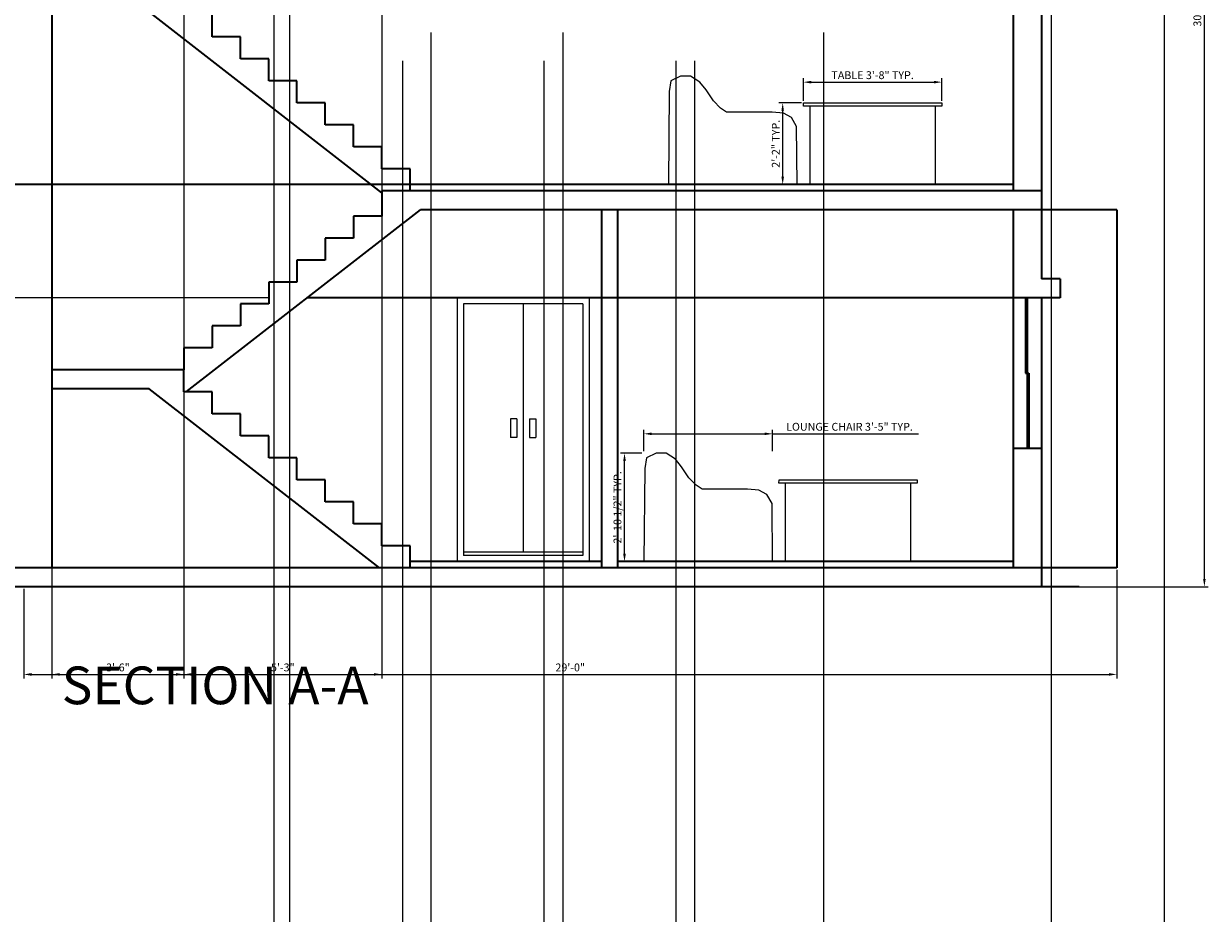
# Model space of a CAD drawing. Units: inches. Extents: x 2443635 to 2446153, y 1826255 to 1827341.
# Tile 13 of 16: x 2445143 to 2445520, y 1826759 to 1827042. Entities that reach past the tile are written whole.
import ezdxf

# ---------------------------------------------------------------- set-up
doc = ezdxf.new("R2010")
doc.units = ezdxf.units.IN
for name, color, linetype, lineweight in [('A-ANNO-LEVL', 4, 'Continuous', 18), ('A-DIMS', 1, 'Continuous', 18), ('A-FURN', 6, 'Continuous', 18), ('A-REFR', 8, 'Continuous', 13), ('A-SECT', 7, 'Continuous', 35), ('A-SECT-PROJ', 9, 'Continuous', 18), ('A-TEXT', 4, 'Continuous', 25)]:
    doc.layers.add(name, color=color, linetype=linetype, lineweight=lineweight)
doc.styles.get("Standard").update_dxf_attribs({"font": 'arial.ttf'})
doc.dimstyles.new('ISO-25', dxfattribs={"dimtxt": 2.5, "dimasz": 2.5, "dimexe": 1.25, "dimexo": 0.625, "dimtad": 1, "dimlunit": 4, "dimtxsty": 'Standard', "dimcen": 2.5, "dimadec": 0, "dimazin": 0, "dimtfac": 1, "dimtmove": 0, "dimatfit": 3, "dimfxl": 1, "dimarcsym": 0})

# ---------------------------------------------------------------- blocks, each defined once
blk = doc.blocks.new('TABLE-SECTION')
at = {"transparency": 33554687}
for p, q in [((2.02, 25), (2.02, 0)), ((42.02, 0), (42.02, 25)), ((2.02, 0), (42.02, 0))]:
    blk.add_line(p, q, dxfattribs=at)
blk.add_lwpolyline([(42.02, 25), (2.02, 25), (0, 25), (0.02, 26), (44.02, 26), (44.06, 25)], close=True, dxfattribs=at)
blk = doc.blocks.new('LOUNGE-CHAIR-SECTION')
at = {"transparency": 33554687}
blk.add_lwpolyline([(0, 0.15), (41.01, 0), (40.81, 18.51), (39.18, 21.33), (36.62, 22.78), (33.02, 23.03), (18.53, 23.09), (16.64, 24.31), (14.33, 26.66), (12.01, 30.12), (10.03, 32.62), (7.07, 34.53), (3.89, 34.53), (0.84, 32.99), (0.3, 29.59), (0.04, 0.15)], dxfattribs=at)
blk = doc.blocks.new('*D74')
at = {"layer": 'A-DIMS', "color": 0, "lineweight": -2, "transparency": 16777216}
for p, q in [((2445391.11, 1827017.33), (2445391.11, 1827024.56)), ((2445435.17, 1827017.33), (2445435.17, 1827024.56)), ((2445393.61, 1827023.31), (2445432.67, 1827023.31))]:
    blk.add_line(p, q, dxfattribs=at)
at = {"layer": 'A-DIMS', "color": 0, "transparency": 16777216}
for points in [[(2445393.61, 1827023.73), (2445393.61, 1827022.89), (2445391.11, 1827023.31)], [(2445432.67, 1827023.73), (2445432.67, 1827022.89), (2445435.17, 1827023.31)]]:
    blk.add_solid(points, dxfattribs=at)
at = {"layer": 'Defpoints', "color": 0, "transparency": 16777216}
for p in [(2445435.17, 1827023.31), (2445391.11, 1827016.7), (2445435.17, 1827016.7)]:
    blk.add_point(p, dxfattribs=at)
at = {"layer": 'A-DIMS', "color": 0, "transparency": 16777216, "insert": (2445413.14, 1827025.21), "char_height": 2.5, "attachment_point": 5}
blk.add_mtext('TABLE 3\'-8" TYP.', dxfattribs=at)
blk = doc.blocks.new('*D75')
at = {"layer": 'A-DIMS', "color": 0, "lineweight": -2, "transparency": 16777216}
for p, q in [((2445390.49, 1827016.7), (2445383.26, 1827016.7)), ((2445384.51, 1826993.2), (2445384.51, 1827014.2)), ((2445390.49, 1826990.7), (2445383.26, 1826990.7))]:
    blk.add_line(p, q, dxfattribs=at)
at = {"layer": 'A-DIMS', "color": 0, "transparency": 16777216}
for points in [[(2445384.09, 1827014.2), (2445384.92, 1827014.2), (2445384.51, 1827016.7)], [(2445384.09, 1826993.2), (2445384.92, 1826993.2), (2445384.51, 1826990.7)]]:
    blk.add_solid(points, dxfattribs=at)
at = {"layer": 'Defpoints', "color": 0, "transparency": 16777216}
for p in [(2445384.51, 1827016.7), (2445391.11, 1827016.7), (2445391.11, 1826990.7)]:
    blk.add_point(p, dxfattribs=at)
at = {"layer": 'A-DIMS', "color": 0, "transparency": 16777216, "insert": (2445382.63, 1827003.7), "char_height": 2.5, "attachment_point": 5, "rotation": 90}
blk.add_mtext('2\'-2" TYP.', dxfattribs=at)
blk = doc.blocks.new('*D88')
at = {"layer": 'A-DIMS', "color": 0, "lineweight": -2, "transparency": 16777216}
for p, q in [((2445340.3, 1826905.86), (2445340.3, 1826912.63)), ((2445342.8, 1826911.38), (2445378.81, 1826911.38)), ((2445381.31, 1826905.86), (2445381.31, 1826912.63)), ((2445381.31, 1826911.38), (2445427.75, 1826911.38))]:
    blk.add_line(p, q, dxfattribs=at)
at = {"layer": 'A-DIMS', "color": 0, "transparency": 16777216}
for points in [[(2445342.8, 1826911.8), (2445342.8, 1826910.97), (2445340.3, 1826911.38)], [(2445378.81, 1826911.8), (2445378.81, 1826910.97), (2445381.31, 1826911.38)]]:
    blk.add_solid(points, dxfattribs=at)
at = {"layer": 'Defpoints', "color": 0, "transparency": 16777216}
for p in [(2445381.31, 1826911.38), (2445340.3, 1826905.23), (2445381.31, 1826905.23)]:
    blk.add_point(p, dxfattribs=at)
at = {"layer": 'A-DIMS', "color": 0, "transparency": 16777216, "insert": (2445405.78, 1826913.3), "char_height": 2.5, "attachment_point": 5}
blk.add_mtext('LOUNGE CHAIR 3\'-5" TYP.', dxfattribs=at)
blk = doc.blocks.new('*D89')
at = {"layer": 'A-DIMS', "color": 0, "lineweight": -2, "transparency": 16777216}
for p, q in [((2445339.68, 1826905.23), (2445332.9, 1826905.23)), ((2445334.15, 1826873.2), (2445334.15, 1826902.73)), ((2445339.68, 1826870.7), (2445332.9, 1826870.7))]:
    blk.add_line(p, q, dxfattribs=at)
at = {"layer": 'A-DIMS', "color": 0, "transparency": 16777216}
for points in [[(2445333.73, 1826902.73), (2445334.57, 1826902.73), (2445334.15, 1826905.23)], [(2445333.73, 1826873.2), (2445334.57, 1826873.2), (2445334.15, 1826870.7)]]:
    blk.add_solid(points, dxfattribs=at)
at = {"layer": 'Defpoints', "color": 0, "transparency": 16777216}
for p in [(2445334.15, 1826905.23), (2445340.3, 1826905.23), (2445340.3, 1826870.7)]:
    blk.add_point(p, dxfattribs=at)
at = {"layer": 'A-DIMS', "color": 0, "transparency": 16777216, "insert": (2445332.23, 1826887.97), "char_height": 2.5, "attachment_point": 5, "rotation": 90}
blk.add_mtext('2\'-10 1/2" TYP.', dxfattribs=at)
blk = doc.blocks.new('*D99')
at = {"layer": 'A-DIMS', "color": 0, "lineweight": -2, "transparency": 16777216}
for p, q in [((2445286.12, 1827228.7), (2445520.01, 1827228.7)), ((2445518.76, 1826865.2), (2445518.76, 1827226.2)), ((2445143.49, 1826862.7), (2445520.01, 1826862.7))]:
    blk.add_line(p, q, dxfattribs=at)
at = {"layer": 'A-DIMS', "color": 0, "transparency": 16777216}
for points in [[(2445518.35, 1827226.2), (2445519.18, 1827226.2), (2445518.76, 1827228.7)], [(2445518.35, 1826865.2), (2445519.18, 1826865.2), (2445518.76, 1826862.7)]]:
    blk.add_solid(points, dxfattribs=at)
at = {"layer": 'Defpoints', "color": 0, "transparency": 16777216}
for p in [(2445285.49, 1827228.7), (2445518.76, 1827228.7), (2445142.86, 1826862.7)]:
    blk.add_point(p, dxfattribs=at)
at = {"layer": 'A-DIMS', "color": 0, "transparency": 16777216, "insert": (2445516.86, 1827045.7), "char_height": 2.5, "attachment_point": 5, "rotation": 90}
blk.add_mtext('30\'-6"', dxfattribs=at)
blk = doc.blocks.new('*D100')
at = {"layer": 'A-DIMS', "color": 0, "lineweight": -2, "transparency": 16777216}
for p, q in [((2445490.86, 1826868.08), (2445490.86, 1826833.55)), ((2445142.86, 1826862.08), (2445142.86, 1826833.55)), ((2445145.36, 1826834.8), (2445488.36, 1826834.8))]:
    blk.add_line(p, q, dxfattribs=at)
at = {"layer": 'A-DIMS', "color": 0, "transparency": 16777216}
for points in [[(2445145.36, 1826835.22), (2445145.36, 1826834.38), (2445142.86, 1826834.8)], [(2445488.36, 1826835.22), (2445488.36, 1826834.38), (2445490.86, 1826834.8)]]:
    blk.add_solid(points, dxfattribs=at)
at = {"layer": 'Defpoints', "color": 0, "transparency": 16777216}
for p in [(2445490.86, 1826868.7), (2445142.86, 1826862.7), (2445490.86, 1826834.8)]:
    blk.add_point(p, dxfattribs=at)
at = {"layer": 'A-DIMS', "color": 0, "transparency": 16777216, "insert": (2445316.86, 1826836.7), "char_height": 2.5, "attachment_point": 5}
blk.add_mtext('29\'-0"', dxfattribs=at)
blk = doc.blocks.new('*D102')
at = {"layer": 'A-DIMS', "color": 0, "lineweight": -2, "transparency": 16777216}
for p, q in [((2445151.86, 1827051.08), (2445151.86, 1826833.55)), ((2445193.86, 1827051.08), (2445193.86, 1826833.55)), ((2445154.36, 1826834.8), (2445191.36, 1826834.8))]:
    blk.add_line(p, q, dxfattribs=at)
at = {"layer": 'A-DIMS', "color": 0, "transparency": 16777216}
for points in [[(2445154.36, 1826835.22), (2445154.36, 1826834.38), (2445151.86, 1826834.8)], [(2445191.36, 1826835.22), (2445191.36, 1826834.38), (2445193.86, 1826834.8)]]:
    blk.add_solid(points, dxfattribs=at)
at = {"layer": 'Defpoints', "color": 0, "transparency": 16777216}
for p in [(2445151.86, 1827051.7), (2445193.86, 1827051.7), (2445193.86, 1826834.8)]:
    blk.add_point(p, dxfattribs=at)
at = {"layer": 'A-DIMS', "color": 0, "transparency": 16777216, "insert": (2445172.86, 1826836.7), "char_height": 2.5, "attachment_point": 5}
blk.add_mtext('3\'-6"', dxfattribs=at)
blk = doc.blocks.new('*D103')
at = {"layer": 'A-DIMS', "color": 0, "lineweight": -2, "transparency": 16777216}
for p, q in [((2445256.86, 1827108.08), (2445256.86, 1826833.55)), ((2445193.86, 1827051.08), (2445193.86, 1826833.55)), ((2445196.36, 1826834.8), (2445254.36, 1826834.8))]:
    blk.add_line(p, q, dxfattribs=at)
at = {"layer": 'A-DIMS', "color": 0, "transparency": 16777216}
for points in [[(2445196.36, 1826835.22), (2445196.36, 1826834.38), (2445193.86, 1826834.8)], [(2445254.36, 1826835.22), (2445254.36, 1826834.38), (2445256.86, 1826834.8)]]:
    blk.add_solid(points, dxfattribs=at)
at = {"layer": 'Defpoints', "color": 0, "transparency": 16777216}
for p in [(2445256.86, 1827108.7), (2445193.86, 1827051.7), (2445256.86, 1826834.8)]:
    blk.add_point(p, dxfattribs=at)
at = {"layer": 'A-DIMS', "color": 0, "transparency": 16777216, "insert": (2445225.36, 1826836.7), "char_height": 2.5, "attachment_point": 5}
blk.add_mtext('5\'-3"', dxfattribs=at)

msp = doc.modelspace()

# ---------------------------------------------------------------- linework, layer by layer
at = {"layer": 'A-ANNO-LEVL'}
msp.add_line((2445220.864, 1826954.701), (2445021.398, 1826954.701), dxfattribs=at)
at = {"layer": 'A-REFR'}
for p, q in [((2445469.966, 1827104.133), (2445469.966, 1826329.288)), ((2445505.966, 1827104.133), (2445505.966, 1826329.288)), ((2445272.466, 1827039.133), (2445272.466, 1826255.288)), ((2445314.466, 1827039.133), (2445314.466, 1826255.288)), ((2445397.466, 1827039.133), (2445397.466, 1826264.288)), ((2445263.466, 1827030.133), (2445263.466, 1826255.288)), ((2445308.466, 1827030.133), (2445308.466, 1826255.288)), ((2445350.466, 1827030.133), (2445350.466, 1826255.288)), ((2445356.466, 1827030.133), (2445356.466, 1826255.288))]:
    msp.add_line(p, q, dxfattribs=at)
at = {"layer": 'A-REFR', "transparency": 33554687}
for p in [(2445227.466, 1827321.207), (2445222.466, 1827316.303)]:
    msp.add_ray(p, (0, -1), dxfattribs=at)
at = {"layer": 'A-SECT'}
for p, q in [((2445151.864, 1827222.701), (2445151.864, 1826868.701)), ((2445457.864, 1827102.701), (2445457.864, 1826988.701)), ((2445466.864, 1827102.701), (2445466.864, 1826982.701)), ((2445256.864, 1826988.1), (2445182.805, 1827045.701)), ((2445202.864, 1827037.701), (2445202.864, 1827044.701)), ((2445211.864, 1827037.701), (2445202.864, 1827037.701)), ((2445211.864, 1827030.701), (2445211.864, 1827037.701)), ((2445220.864, 1827030.701), (2445211.864, 1827030.701)), ((2445220.864, 1827023.701), (2445220.864, 1827030.701)), ((2445229.864, 1827023.701), (2445220.864, 1827023.701)), ((2445229.864, 1827016.701), (2445229.864, 1827023.701)), ((2445238.864, 1827016.701), (2445229.864, 1827016.701)), ((2445238.864, 1827009.701), (2445238.864, 1827016.701)), ((2445247.864, 1827009.701), (2445238.864, 1827009.701)), ((2445247.864, 1827002.701), (2445247.864, 1827009.701)), ((2445256.864, 1827002.701), (2445247.864, 1827002.701)), ((2445256.864, 1826995.701), (2445256.864, 1827002.701)), ((2445265.864, 1826995.701), (2445256.864, 1826995.701)), ((2445265.864, 1826988.701), (2445265.864, 1826995.701)), ((2445457.864, 1826990.701), (2445021.398, 1826990.701)), ((2445466.864, 1826988.701), (2445256.864, 1826988.701)), ((2445256.864, 1826988.701), (2445256.864, 1826980.701)), ((2445194.637, 1826924.701), (2445269.208, 1826982.701)), ((2445490.864, 1826982.701), (2445269.208, 1826982.701)), ((2445326.864, 1826982.701), (2445326.864, 1826868.701)), ((2445331.864, 1826982.701), (2445331.864, 1826868.701)), ((2445457.864, 1826982.701), (2445457.864, 1826868.701)), ((2445466.864, 1826982.701), (2445466.864, 1826960.701)), ((2445490.864, 1826982.701), (2445490.864, 1826868.701)), ((2445256.864, 1826980.701), (2445247.864, 1826980.701)), ((2445247.864, 1826980.701), (2445247.864, 1826973.701)), ((2445247.864, 1826973.701), (2445238.864, 1826973.701)), ((2445238.864, 1826973.701), (2445238.864, 1826966.701)), ((2445238.864, 1826966.701), (2445229.864, 1826966.701)), ((2445229.864, 1826966.701), (2445229.864, 1826959.701)), ((2445472.864, 1826960.701), (2445466.864, 1826960.701)), ((2445472.864, 1826960.701), (2445472.864, 1826954.701)), ((2445229.864, 1826959.701), (2445220.864, 1826959.701)), ((2445220.864, 1826959.701), (2445220.864, 1826952.701)), ((2445220.864, 1826952.701), (2445211.864, 1826952.701)), ((2445211.864, 1826952.701), (2445211.864, 1826945.701)), ((2445457.864, 1826954.701), (2445233.208, 1826954.701)), ((2445472.864, 1826954.701), (2445457.864, 1826954.701)), ((2445461.864, 1826954.701), (2445461.864, 1826930.701)), ((2445462.364, 1826954.701), (2445462.364, 1826906.701)), ((2445466.864, 1826954.701), (2445466.864, 1826862.701)), ((2445211.864, 1826945.701), (2445202.864, 1826945.701)), ((2445202.864, 1826945.701), (2445202.864, 1826938.701)), ((2445202.864, 1826938.701), (2445193.864, 1826938.701)), ((2445193.864, 1826938.701), (2445193.864, 1826931.701)), ((2445193.864, 1826931.701), (2445151.864, 1826931.701)), ((2445193.864, 1826931.701), (2445151.864, 1826931.701)), ((2445193.864, 1826924.701), (2445193.864, 1826931.701)), ((2445461.864, 1826930.701), (2445462.864, 1826930.701)), ((2445462.864, 1826930.701), (2445462.864, 1826906.701)), ((2445182.805, 1826925.701), (2445151.864, 1826925.701)), ((2445256.091, 1826868.701), (2445182.805, 1826925.701)), ((2445202.864, 1826924.701), (2445193.864, 1826924.701)), ((2445202.864, 1826917.701), (2445202.864, 1826924.701)), ((2445211.864, 1826917.701), (2445202.864, 1826917.701)), ((2445211.864, 1826910.701), (2445211.864, 1826917.701)), ((2445220.864, 1826910.701), (2445211.864, 1826910.701)), ((2445220.864, 1826903.701), (2445220.864, 1826910.701)), ((2445229.864, 1826903.701), (2445220.864, 1826903.701)), ((2445229.864, 1826896.701), (2445229.864, 1826903.701)), ((2445466.864, 1826906.701), (2445457.864, 1826906.701)), ((2445238.864, 1826896.701), (2445229.864, 1826896.701)), ((2445238.864, 1826889.701), (2445238.864, 1826896.701)), ((2445247.864, 1826889.701), (2445238.864, 1826889.701)), ((2445247.864, 1826882.701), (2445247.864, 1826889.701)), ((2445256.864, 1826882.701), (2445247.864, 1826882.701)), ((2445256.864, 1826875.701), (2445256.864, 1826882.701)), ((2445265.864, 1826875.701), (2445256.864, 1826875.701)), ((2445265.864, 1826868.701), (2445265.864, 1826875.701)), ((2445326.864, 1826870.701), (2445265.864, 1826870.701)), ((2445457.864, 1826870.701), (2445331.864, 1826870.701)), ((2445490.864, 1826868.701), (2445021.398, 1826868.701)), ((2445478.864, 1826862.701), (2445021.398, 1826862.701))]:
    msp.add_line(p, q, dxfattribs=at)
at = {"layer": 'A-SECT-PROJ'}
for p, q in [((2445280.864, 1826954.701), (2445280.864, 1826870.701)), ((2445322.864, 1826954.701), (2445280.864, 1826954.701)), ((2445320.864, 1826952.701), (2445282.864, 1826952.701)), ((2445282.864, 1826952.701), (2445282.864, 1826872.701)), ((2445301.864, 1826952.701), (2445301.864, 1826873.701)), ((2445320.864, 1826952.701), (2445320.864, 1826872.701)), ((2445322.864, 1826954.701), (2445322.864, 1826870.701)), ((2445297.864, 1826916.201), (2445297.864, 1826910.201)), ((2445299.864, 1826916.201), (2445297.864, 1826916.201)), ((2445299.864, 1826916.201), (2445299.864, 1826910.201)), ((2445303.864, 1826916.201), (2445303.864, 1826910.201)), ((2445303.864, 1826916.201), (2445305.864, 1826916.201)), ((2445305.864, 1826916.201), (2445305.864, 1826910.201)), ((2445299.864, 1826910.201), (2445297.864, 1826910.201)), ((2445303.864, 1826910.201), (2445305.864, 1826910.201)), ((2445320.864, 1826873.701), (2445282.864, 1826873.701)), ((2445322.864, 1826870.701), (2445280.864, 1826870.701)), ((2445320.864, 1826872.701), (2445282.864, 1826872.701))]:
    msp.add_line(p, q, dxfattribs=at)

# ---------------------------------------------------------------- block references
at = {"layer": 'A-FURN', "transparency": 33554687}
for name, p in [('LOUNGE-CHAIR-SECTION', (2445348.104, 1826990.701)), ('TABLE-SECTION', (2445391.115, 1826990.701)), ('LOUNGE-CHAIR-SECTION', (2445340.303, 1826870.701)), ('TABLE-SECTION', (2445383.314, 1826870.701))]:
    msp.add_blockref(name, p, dxfattribs=at)

# ---------------------------------------------------------------- texts
at = {"layer": 'A-TEXT', "transparency": 33554687, "insert": (2445154.983, 1826837.315), "char_height": 12, "attachment_point": 1}
msp.add_mtext_dynamic_manual_height_columns('SECTION A-A', width=201.69861, gutter_width=12.5, heights=[0], dxfattribs=at)

# ---------------------------------------------------------------- dimensions: what is measured, and where the dimension line sits
at = {"layer": 'A-DIMS', "transparency": 33554687}
dim = msp.add_linear_dim(base=(2445518.764, 1827228.701), p1=(2445142.864, 1826862.701), p2=(2445285.491, 1827228.701), angle=90, dimstyle='ISO-25', override={"dimdec": 1, "dimlfac": 1, "dimrnd": 0, "dimzin": 1, "dimdsep": 46, "dimlunit": 4, "dimfrac": 2}, dxfattribs=at)
dim.commit()
dim.dimension.update_dxf_attribs({"geometry": '*D99', "text_midpoint": (2445516.861, 1827045.701)})
for base, p1, p2, picture, middle in [((2445256.864, 1826834.801), (2445193.864, 1827051.701), (2445256.864, 1827108.701), '*D103', (2445225.364, 1826836.703)), ((2445193.864, 1826834.801), (2445151.864, 1827051.701), (2445193.864, 1827051.701), '*D102', (2445172.864, 1826836.703)), ((2445490.864, 1826834.801), (2445142.864, 1826862.701), (2445490.864, 1826868.701), '*D100', (2445316.864, 1826836.703))]:
    dim = msp.add_linear_dim(base=base, p1=p1, p2=p2, dimstyle='ISO-25', override={"dimdec": 1, "dimlfac": 1, "dimrnd": 0, "dimzin": 1, "dimdsep": 46, "dimlunit": 4, "dimfrac": 2}, dxfattribs=at)
    dim.commit()
    dim.dimension.update_dxf_attribs({"geometry": picture, "text_midpoint": middle})
for base, p1, p2, text, picture, middle in [((2445435.172, 1827023.31), (2445391.115, 1827016.701), (2445435.172, 1827016.701), 'TABLE <> TYP.', '*D74', (2445413.144, 1827025.212)), ((2445381.314, 1826911.384), (2445340.303, 1826905.232), (2445381.314, 1826905.232), 'LOUNGE CHAIR <> TYP.', '*D88', (2445405.782, 1826913.303))]:
    dim = msp.add_linear_dim(base=base, p1=p1, p2=p2, text=text, dimstyle='ISO-25', override={"dimdec": 1, "dimlfac": 1, "dimrnd": 0, "dimzin": 1, "dimdsep": 46, "dimlunit": 4, "dimfrac": 2}, dxfattribs=at)
    dim.commit()
    dim.dimension.update_dxf_attribs({"geometry": picture, "text_midpoint": middle})
for base, p1, p2, picture, middle in [((2445384.506, 1827016.701), (2445391.115, 1826990.701), (2445391.115, 1827016.701), '*D75', (2445382.625, 1827003.701)), ((2445334.152, 1826905.232), (2445340.303, 1826870.701), (2445340.303, 1826905.232), '*D89', (2445332.234, 1826887.967))]:
    dim = msp.add_linear_dim(base=base, p1=p1, p2=p2, angle=90, text='<> TYP.', dimstyle='ISO-25', override={"dimdec": 1, "dimlfac": 1, "dimrnd": 0, "dimzin": 1, "dimdsep": 46, "dimlunit": 4, "dimfrac": 2}, dxfattribs=at)
    dim.commit()
    dim.dimension.update_dxf_attribs({"geometry": picture, "text_midpoint": middle})

doc.saveas('drawing.dxf')
